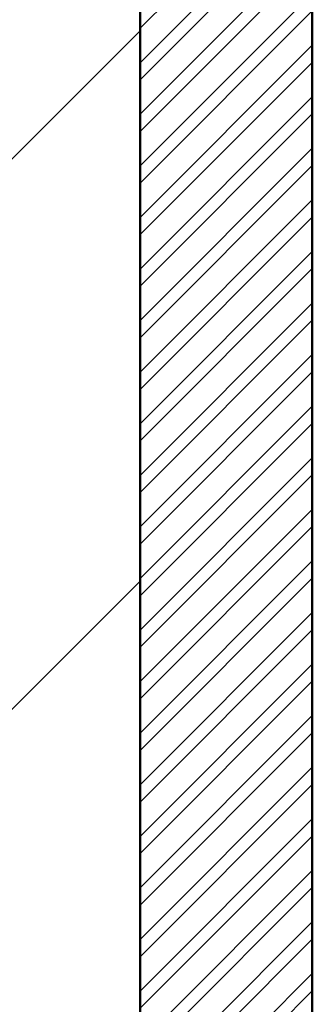
# Model space of a CAD drawing. Units: inches. Extents: x 3590 to 5167, y 65 to 1917.
# Tile 61 of 100: x 5065 to 5080, y 1558 to 1609. Entities that reach past the tile are written whole.
import ezdxf

# ---------------------------------------------------------------- set-up
doc = ezdxf.new("R2010")
doc.units = ezdxf.units.IN
for name, color, linetype, lineweight in [('A-FLOR-PATT', 8, 'Continuous', 13), ('A-WALL', 7, 'Continuous', 50), ('A-WALL-PATT', 251, 'Continuous', 13)]:
    doc.layers.add(name, color=color, linetype=linetype, lineweight=lineweight)

msp = doc.modelspace()

# ---------------------------------------------------------------- hatches: boundary and pattern name
at = {"layer": 'A-FLOR-PATT', "transparency": 33554687}
h = msp.add_hatch(dxfattribs=at)
h.set_pattern_fill('AR-HBONE', color=256, scale=0.2)
h.set_pattern_definition([(45, (-588.972, 0), (0, 28.73682), [60.96, -20.32]), (135, (-574.604, 14.368), (3e-15, 28.73682), [60.96, -20.32])])
h.paths.add_polyline_path([(5071.274, 1796.999), (4933.274, 1796.999), (4933.274, 1753.999), (4962.774, 1753.999, -0.414214), (4928.774, 1719.999), (4933.274, 1718.999), (4933.274, 1334.999), (5071.274, 1334.999)])
h.paths.add_polyline_path([(4951.78, 1521.077), (4951.715, 1521.04), (4951.563, 1520.895)], flags=16)
h.paths.add_polyline_path([(4952.267, 1521.376), (4952.198, 1521.371), (4952.198, 1521.356)], flags=0)
h.paths.add_polyline_path([(4967.051, 1529.728), (4965.231, 1528.694), (4963.411, 1527.714), (4961.756, 1526.851), (4963.589, 1527.449), (4964.036, 1527.478), (4962.975, 1527.249), (4961.76, 1526.852), (4959.792, 1525.834), (4958.005, 1524.895), (4956.24, 1523.93), (4954.504, 1522.919), (4954.129, 1522.682), (4953.361, 1521.997), (4953.366, 1521.998), (4953.605, 1522.064), (4955.106, 1522.761), (4956.921, 1523.434), (4958.678, 1523.915), (4960.358, 1524.2), (4961.945, 1524.286), (4964.171, 1524.108), (4965.958, 1523.309), (4963.863, 1522.976), (4965.187, 1522.499), (4963.366, 1522.497), (4961.545, 1522.487), (4959.764, 1522.461), (4958.304, 1522.419), (4957.974, 1522.388), (4956.307, 1522.232), (4954.718, 1522.071), (4953.251, 1521.899), (4953.525, 1521.623), (4954.331, 1521.379), (4956.243, 1521.23), (4958.039, 1520.93), (4959.684, 1520.483), (4961.16, 1519.896), (4963.107, 1518.8), (4964.393, 1517.325), (4962.973, 1517.726), (4964.558, 1516.661), (4965.407, 1515.708), (4963.507, 1516.322), (4961.68, 1517.005), (4959.935, 1517.745), (4958.282, 1518.528), (4956.732, 1519.343), (4955.295, 1520.175), (4954.672, 1520.572), (4954.513, 1520.627), (4955.658, 1519.318), (4956.703, 1517.982), (4957.644, 1516.647), (4958.485, 1515.334), (4959.55, 1513.524), (4960.438, 1511.769), (4958.841, 1513.62), (4957.452, 1515.325), (4955.819, 1517.459), (4956.665, 1515.448), (4957.111, 1513.923), (4957.447, 1511.714), (4957.076, 1509.793), (4956.538, 1511.11), (4955.992, 1512.569), (4955.444, 1514.125), (4954.898, 1515.735), (4954.357, 1517.356), (4953.824, 1518.943), (4953.305, 1520.452), (4953.065, 1521.116), (4952.971, 1521.146), (4952.949, 1521.086), (4952.73, 1520.199), (4953.37, 1518.024), (4953.757, 1516.373), (4954.051, 1514.765), (4954.264, 1513.221), (4954.471, 1511.131), (4954.497, 1510.402), (4954.409, 1511.76), (4954.264, 1513.221), (4954.051, 1514.765), (4953.757, 1516.373), (4953.37, 1518.024), (4952.877, 1519.698), (4952.716, 1520.141), (4952.533, 1519.059), (4952.374, 1517.789), (4952.219, 1516.312), (4952.046, 1514.6), (4951.833, 1512.626), (4951.557, 1510.363), (4951.203, 1512.168), (4950.852, 1514.339), (4950.985, 1516.376), (4951.66, 1518.286), (4952.593, 1520.481), (4952.357, 1521.13), (4951.855, 1520.328), (4950.839, 1518.908), (4949.777, 1517.587), (4948.916, 1516.617), (4948.111, 1515.256), (4947.089, 1513.554), (4945.889, 1511.615), (4946.326, 1513.402), (4946.562, 1514.249), (4945.528, 1513.327), (4944.581, 1512.531), (4946.018, 1514.508), (4947.204, 1516.048), (4947.893, 1517.313), (4949.307, 1518.764), (4950.414, 1519.767), (4950.451, 1519.806), (4952.267, 1521.376), (4951.645, 1521.493), (4950.404, 1521.18), (4948.044, 1520.359), (4946.119, 1519.452), (4944.572, 1518.475), (4943.35, 1517.443), (4941.997, 1515.92), (4941.661, 1515.275), (4942.813, 1516.99), (4944.572, 1518.475), (4946.119, 1519.452), (4948.044, 1520.359), (4950.404, 1521.18), (4951.645, 1521.493), (4949.647, 1521.868), (4948.6, 1521.756), (4947.126, 1521.57), (4945.42, 1521.348), (4943.45, 1521.105), (4941.183, 1520.856), (4942.86, 1521.613), (4943.873, 1522.03), (4942.952, 1521.909), (4941.41, 1521.485), (4939.543, 1520.67), (4938.968, 1520.226), (4940.733, 1521.299), (4942.952, 1521.909), (4943.702, 1522.008), (4945.894, 1522.7), (4947.565, 1522.714), (4948.921, 1522.566), (4951.131, 1522.183), (4950.971, 1522.297), (4948.129, 1523.006), (4946.035, 1523.707), (4944.232, 1524.521), (4942.707, 1525.461), (4941.444, 1526.537), (4940.43, 1527.761), (4939.649, 1529.143), (4941.421, 1528.122), (4943.147, 1527.132), (4944.841, 1526.175), (4946.514, 1525.25), (4948.179, 1524.359), (4948.365, 1524.263), (4946.475, 1526.045), (4945.181, 1527.54), (4944.19, 1529.033), (4943.496, 1530.54), (4943.278, 1531.36), (4942.498, 1531.919), (4943.114, 1531.762), (4942.959, 1533.659), (4944.14, 1531.989), (4944.612, 1531.323), (4946.202, 1530.463), (4947.486, 1529.509), (4948.79, 1528.226), (4950.368, 1526.237), (4949.485, 1528.155), (4948.851, 1530.123), (4948.491, 1532.041), (4948.381, 1533.918), (4948.501, 1535.76), (4948.827, 1537.573), (4949.418, 1535.565), (4949.957, 1533.569), (4950.464, 1531.586), (4950.961, 1529.617), (4951.391, 1527.954), (4951.724, 1530.687), (4952.201, 1532.58), (4952.889, 1534.33), (4953.77, 1535.951), (4954.827, 1537.46), (4954.521, 1535.39), (4954.273, 1533.937), (4955.58, 1535.663), (4956.748, 1536.739), (4956.159, 1534.78), (4955.589, 1532.873), (4955.043, 1531.006), (4954.525, 1529.166), (4954.038, 1527.341), (4953.638, 1525.733), (4953.611, 1525.586), (4953.398, 1524.166), (4953.382, 1524.009), (4954.07, 1525.476), (4954.912, 1527.022), (4956.136, 1528.894), (4957.847, 1530.577), (4959.376, 1531.54), (4958.256, 1530.104), (4957.143, 1528.663), (4956.066, 1527.243), (4955.056, 1525.871), (4954.141, 1524.571), (4953.352, 1523.372), (4953.311, 1523.303), (4953.273, 1522.925), (4953.261, 1522.382), (4954.103, 1523.373), (4954.63, 1524.284), (4955.961, 1526.358), (4957.23, 1528.13), (4958.421, 1529.609), (4960.037, 1531.368), (4961.374, 1532.375), (4962.101, 1532.77), (4961.07, 1531.061), (4959.987, 1529.438), (4958.869, 1527.908), (4958.15, 1527.007), (4959.803, 1528.003), (4961.589, 1528.793), (4963.391, 1529.328), (4965.211, 1529.632)], flags=16)
h.paths.add_polyline_path([(4962.944, 1523.182), (4961.107, 1523.422), (4960.392, 1523.362), (4962.35, 1523.331)], flags=0)
h.paths.add_polyline_path([(5049.541, 1584.551), (5049.476, 1584.515), (5049.325, 1584.37)], flags=16)
h.paths.add_polyline_path([(5050.028, 1584.851), (5049.959, 1584.845), (5049.959, 1584.83)], flags=0)
h.paths.add_polyline_path([(5042.333, 1581.949), (5043.88, 1582.926), (5045.806, 1583.833), (5048.165, 1584.654), (5049.406, 1584.967), (5047.408, 1585.342), (5046.361, 1585.231), (5044.888, 1585.044), (5043.181, 1584.822), (5041.211, 1584.579), (5038.944, 1584.33), (5040.622, 1585.087), (5041.634, 1585.504), (5040.713, 1585.383), (5039.171, 1584.959), (5037.304, 1584.144), (5036.729, 1583.7), (5038.494, 1584.773), (5040.713, 1585.383), (5041.463, 1585.482), (5043.655, 1586.174), (5045.326, 1586.188), (5046.682, 1586.04), (5048.893, 1585.657), (5048.732, 1585.771), (5045.891, 1586.48), (5043.796, 1587.181), (5041.994, 1587.996), (5040.468, 1588.935), (5039.205, 1590.011), (5038.191, 1591.235), (5037.41, 1592.617), (5039.182, 1591.596), (5040.909, 1590.607), (5042.602, 1589.649), (5044.275, 1588.724), (5045.94, 1587.833), (5046.126, 1587.738), (5044.237, 1589.519), (5042.942, 1591.015), (5041.952, 1592.508), (5041.257, 1594.014), (5041.039, 1594.834), (5040.26, 1595.393), (5040.875, 1595.237), (5040.721, 1597.133), (5041.901, 1595.463), (5042.373, 1594.798), (5043.963, 1593.938), (5045.247, 1592.983), (5046.552, 1591.701), (5048.129, 1589.712), (5047.247, 1591.63), (5046.613, 1593.597), (5046.252, 1595.515), (5046.142, 1597.392), (5046.262, 1599.234), (5046.588, 1601.047), (5047.179, 1599.039), (5047.718, 1597.043), (5048.225, 1595.06), (5048.722, 1593.091), (5049.152, 1591.429), (5049.485, 1594.161), (5049.962, 1596.054), (5050.65, 1597.804), (5051.532, 1599.425), (5052.589, 1600.934), (5052.283, 1598.864), (5052.034, 1597.411), (5053.341, 1599.137), (5054.509, 1600.213), (5053.92, 1598.254), (5053.35, 1596.348), (5052.805, 1594.48), (5052.286, 1592.64), (5051.799, 1590.815), (5051.4, 1589.207), (5051.373, 1589.06), (5051.159, 1587.64), (5051.143, 1587.483), (5051.831, 1588.95), (5052.673, 1590.496), (5053.898, 1592.368), (5055.608, 1594.051), (5057.137, 1595.014), (5056.017, 1593.578), (5054.904, 1592.137), (5053.828, 1590.717), (5052.817, 1589.345), (5051.902, 1588.046), (5051.113, 1586.846), (5051.072, 1586.777), (5051.034, 1586.399), (5051.022, 1585.856), (5051.864, 1586.847), (5052.391, 1587.758), (5053.723, 1589.832), (5054.991, 1591.604), (5056.182, 1593.083), (5057.798, 1594.842), (5059.135, 1595.849), (5059.863, 1596.244), (5058.831, 1594.535), (5057.749, 1592.912), (5056.63, 1591.382), (5055.912, 1590.482), (5057.564, 1591.477), (5059.35, 1592.267), (5061.152, 1592.802), (5062.972, 1593.106), (5064.812, 1593.203), (5062.992, 1592.169), (5061.172, 1591.188), (5059.518, 1590.325), (5061.35, 1590.924), (5061.797, 1590.952), (5060.737, 1590.723), (5059.521, 1590.326), (5057.553, 1589.308), (5055.766, 1588.369), (5054.002, 1587.404), (5052.265, 1586.393), (5051.891, 1586.156), (5051.122, 1585.471), (5051.127, 1585.472), (5051.366, 1585.538), (5052.867, 1586.235), (5054.682, 1586.908), (5056.439, 1587.389), (5058.12, 1587.675), (5059.706, 1587.76), (5061.933, 1587.583), (5063.719, 1586.783), (5061.624, 1586.45), (5062.949, 1585.973), (5061.127, 1585.971), (5059.307, 1585.961), (5057.525, 1585.935), (5056.065, 1585.893), (5055.735, 1585.862), (5054.068, 1585.707), (5052.479, 1585.546), (5051.012, 1585.373), (5051.286, 1585.097), (5052.092, 1584.853), (5054.004, 1584.704), (5055.8, 1584.404), (5057.446, 1583.958), (5058.921, 1583.37), (5060.868, 1582.274), (5062.154, 1580.799), (5060.734, 1581.2), (5062.32, 1580.135), (5063.168, 1579.182), (5061.269, 1579.796), (5059.441, 1580.479), (5057.696, 1581.219), (5056.043, 1582.003), (5054.493, 1582.817), (5053.057, 1583.649), (5052.433, 1584.047), (5052.274, 1584.101), (5053.42, 1582.793), (5054.464, 1581.457), (5055.405, 1580.121), (5056.247, 1578.809), (5057.311, 1576.998), (5058.199, 1575.244), (5056.602, 1577.094), (5055.213, 1578.799), (5053.58, 1580.933), (5054.427, 1578.922), (5054.872, 1577.397), (5055.208, 1575.189), (5054.838, 1573.267), (5054.299, 1574.584), (5053.754, 1576.043), (5053.206, 1577.599), (5052.659, 1579.209), (5052.118, 1580.83), (5051.585, 1582.417), (5051.066, 1583.927), (5050.826, 1584.59), (5050.733, 1584.62), (5050.711, 1584.561), (5050.491, 1583.673), (5051.131, 1581.498), (5051.518, 1579.847), (5051.813, 1578.24), (5052.026, 1576.695), (5052.233, 1574.605), (5052.258, 1573.876), (5052.17, 1575.234), (5052.026, 1576.695), (5051.813, 1578.24), (5051.518, 1579.847), (5051.131, 1581.498), (5050.638, 1583.172), (5050.477, 1583.615), (5050.294, 1582.533), (5050.136, 1581.263), (5049.981, 1579.786), (5049.807, 1578.074), (5049.594, 1576.1), (5049.318, 1573.837), (5048.965, 1575.642), (5048.613, 1577.813), (5048.747, 1579.85), (5049.421, 1581.76), (5050.354, 1583.955), (5050.118, 1584.604), (5049.616, 1583.802), (5048.6, 1582.382), (5047.538, 1581.061), (5046.677, 1580.091), (5045.872, 1578.73), (5044.85, 1577.028), (5043.651, 1575.089), (5044.087, 1576.877), (5044.324, 1577.723), (5043.289, 1576.801), (5042.342, 1576.005), (5043.779, 1577.982), (5044.966, 1579.522), (5045.655, 1580.787), (5047.068, 1582.239), (5048.175, 1583.241), (5048.213, 1583.28), (5050.028, 1584.851), (5049.406, 1584.967), (5048.165, 1584.654), (5045.806, 1583.833), (5043.88, 1582.926), (5042.333, 1581.949), (5041.111, 1580.917), (5039.758, 1579.394), (5039.423, 1578.749), (5040.575, 1580.464)], flags=16)
h.paths.add_polyline_path([(4954.799, 1533.12), (4954.262, 1532.079), (4953.831, 1530.935), (4953.505, 1529.636), (4953.283, 1528.133), (4953.167, 1526.376), (4953.156, 1524.315), (4953.277, 1521.236), (4952.802, 1521.842), (4951.557, 1521.998), (4950.976, 1521.961), (4952.661, 1521.941), (4952.802, 1521.842), (4953.152, 1523.593), (4953.167, 1526.376), (4953.283, 1528.133), (4953.609, 1530.346), (4954.456, 1532.592)], flags=0)
h.paths.add_polyline_path([(5050.563, 1585.316), (5049.318, 1585.472), (5048.737, 1585.435), (5050.422, 1585.415), (5050.563, 1585.316), (5050.914, 1587.067), (5050.928, 1589.851), (5051.045, 1591.607), (5051.371, 1593.82), (5052.217, 1596.066), (5052.56, 1596.594), (5052.024, 1595.554), (5051.592, 1594.409), (5051.266, 1593.11), (5051.045, 1591.607), (5050.928, 1589.851), (5050.918, 1587.789), (5051.038, 1584.71)], flags=0)
h.paths.add_polyline_path([(5058.153, 1586.836), (5060.111, 1586.805), (5060.705, 1586.656), (5058.868, 1586.896)], flags=0)
h.paths.add_polyline_path([(5049.541, 1430.936), (5049.476, 1430.9), (5049.325, 1430.755)], flags=16)
h.paths.add_polyline_path([(5050.028, 1431.236), (5049.959, 1431.231), (5049.959, 1431.215)], flags=0)
h.paths.add_polyline_path([(5046.588, 1447.432), (5047.179, 1445.425), (5047.718, 1443.429), (5048.225, 1441.446), (5048.722, 1439.476), (5049.152, 1437.814), (5049.485, 1440.546), (5049.962, 1442.439), (5050.65, 1444.189), (5051.532, 1445.811), (5052.589, 1447.319), (5052.283, 1445.249), (5052.034, 1443.796), (5053.341, 1445.522), (5054.509, 1446.598), (5053.92, 1444.64), (5053.35, 1442.733), (5052.805, 1440.865), (5052.286, 1439.025), (5051.799, 1437.201), (5051.4, 1435.592), (5051.373, 1435.445), (5051.159, 1434.025), (5051.143, 1433.868), (5051.831, 1435.335), (5052.673, 1436.881), (5053.898, 1438.753), (5055.608, 1440.436), (5057.137, 1441.4), (5056.017, 1439.963), (5054.904, 1438.522), (5053.828, 1437.102), (5052.817, 1435.73), (5051.902, 1434.431), (5051.113, 1433.231), (5051.072, 1433.162), (5051.034, 1432.784), (5051.022, 1432.242), (5051.864, 1433.232), (5052.391, 1434.143), (5053.723, 1436.217), (5054.991, 1437.989), (5056.182, 1439.468), (5057.798, 1441.227), (5059.135, 1442.235), (5059.863, 1442.629), (5058.831, 1440.921), (5057.749, 1439.298), (5056.63, 1437.767), (5055.912, 1436.867), (5057.564, 1437.863), (5059.35, 1438.652), (5061.152, 1439.187), (5062.972, 1439.491), (5064.812, 1439.588), (5062.992, 1438.554), (5061.172, 1437.573), (5059.518, 1436.71), (5061.35, 1437.309), (5061.797, 1437.337), (5060.737, 1437.108), (5059.521, 1436.711), (5057.553, 1435.693), (5055.766, 1434.754), (5054.002, 1433.789), (5052.265, 1432.778), (5051.891, 1432.541), (5051.122, 1431.856), (5051.127, 1431.857), (5051.366, 1431.923), (5052.867, 1432.62), (5054.682, 1433.293), (5056.439, 1433.775), (5058.12, 1434.06), (5059.706, 1434.145), (5061.933, 1433.968), (5063.719, 1433.168), (5061.624, 1432.835), (5062.949, 1432.358), (5061.127, 1432.357), (5059.307, 1432.346), (5057.525, 1432.32), (5056.065, 1432.278), (5055.735, 1432.248), (5054.068, 1432.092), (5052.479, 1431.931), (5051.012, 1431.759), (5051.286, 1431.482), (5052.092, 1431.238), (5054.004, 1431.089), (5055.8, 1430.789), (5057.446, 1430.343), (5058.921, 1429.755), (5060.868, 1428.66), (5062.154, 1427.185), (5060.734, 1427.585), (5062.32, 1426.52), (5063.168, 1425.567), (5061.269, 1426.181), (5059.441, 1426.865), (5057.696, 1427.604), (5056.043, 1428.388), (5054.493, 1429.202), (5053.057, 1430.034), (5052.433, 1430.432), (5052.274, 1430.487), (5053.42, 1429.178), (5054.464, 1427.842), (5055.405, 1426.506), (5056.247, 1425.194), (5057.311, 1423.383), (5058.199, 1421.629), (5056.602, 1423.479), (5055.213, 1425.184), (5053.58, 1427.318), (5054.427, 1425.307), (5054.872, 1423.782), (5055.208, 1421.574), (5054.838, 1419.652), (5054.299, 1420.97), (5053.754, 1422.428), (5053.206, 1423.984), (5052.659, 1425.595), (5052.118, 1427.215), (5051.585, 1428.802), (5051.066, 1430.312), (5050.826, 1430.975), (5050.733, 1431.005), (5050.711, 1430.946), (5050.491, 1430.058), (5051.131, 1427.883), (5051.518, 1426.232), (5051.813, 1424.625), (5052.026, 1423.081), (5052.233, 1420.991), (5052.258, 1420.261), (5052.17, 1421.619), (5052.026, 1423.081), (5051.813, 1424.625), (5051.518, 1426.232), (5051.131, 1427.883), (5050.638, 1429.558), (5050.477, 1430.001), (5050.294, 1428.918), (5050.136, 1427.648), (5049.981, 1426.171), (5049.807, 1424.459), (5049.594, 1422.485), (5049.318, 1420.222), (5048.965, 1422.028), (5048.613, 1424.199), (5048.747, 1426.235), (5049.421, 1428.146), (5050.354, 1430.34), (5050.118, 1430.989), (5049.616, 1430.187), (5048.6, 1428.768), (5047.538, 1427.446), (5046.677, 1426.477), (5045.872, 1425.116), (5044.85, 1423.413), (5043.651, 1421.474), (5044.087, 1423.262), (5044.324, 1424.109), (5043.289, 1423.186), (5042.342, 1422.391), (5043.779, 1424.368), (5044.966, 1425.907), (5045.655, 1427.173), (5047.068, 1428.624), (5048.175, 1429.627), (5048.213, 1429.666), (5050.028, 1431.236), (5049.406, 1431.353), (5048.165, 1431.039), (5045.806, 1430.218), (5043.88, 1429.311), (5042.333, 1428.334), (5041.111, 1427.302), (5039.758, 1425.779), (5039.423, 1425.134), (5040.575, 1426.849), (5042.333, 1428.334), (5043.88, 1429.311), (5045.806, 1430.218), (5048.165, 1431.039), (5049.406, 1431.353), (5047.408, 1431.727), (5046.361, 1431.616), (5044.888, 1431.429), (5043.181, 1431.207), (5041.211, 1430.964), (5038.944, 1430.715), (5040.622, 1431.472), (5041.634, 1431.89), (5040.713, 1431.769), (5039.171, 1431.345), (5037.304, 1430.53), (5036.729, 1430.085), (5038.494, 1431.158), (5040.713, 1431.769), (5041.463, 1431.867), (5043.655, 1432.559), (5045.326, 1432.573), (5046.682, 1432.425), (5048.893, 1432.042), (5048.732, 1432.156), (5045.891, 1432.865), (5043.796, 1433.566), (5041.994, 1434.381), (5040.468, 1435.321), (5039.205, 1436.396), (5038.191, 1437.62), (5037.41, 1439.002), (5039.182, 1437.982), (5040.909, 1436.992), (5042.602, 1436.034), (5044.275, 1435.109), (5045.94, 1434.218), (5046.126, 1434.123), (5044.237, 1435.904), (5042.942, 1437.4), (5041.952, 1438.893), (5041.257, 1440.399), (5041.039, 1441.219), (5040.26, 1441.778), (5040.875, 1441.622), (5040.721, 1443.518), (5041.901, 1441.848), (5042.373, 1441.183), (5043.963, 1440.323), (5045.247, 1439.369), (5046.552, 1438.086), (5048.129, 1436.097), (5047.247, 1438.015), (5046.613, 1439.982), (5046.252, 1441.901), (5046.142, 1443.778), (5046.262, 1445.619)], flags=16)
h.paths.add_polyline_path([(5052.382, 1444.255), (5051.623, 1442.78), (5052.024, 1441.939), (5052.56, 1442.98)], flags=0)
h.paths.add_polyline_path([(5050.563, 1431.701), (5049.318, 1431.857), (5048.737, 1431.821), (5050.422, 1431.8)], flags=0)
h.paths.add_polyline_path([(5058.153, 1433.221), (5060.111, 1433.19), (5060.705, 1433.041), (5058.868, 1433.281)], flags=0)
h.paths.add_polyline_path([(5049.541, 1352.285), (5049.476, 1352.249), (5049.325, 1352.104)], flags=16)
h.paths.add_polyline_path([(5050.028, 1352.585), (5049.959, 1352.58), (5049.959, 1352.564)], flags=0)
h.paths.add_polyline_path([(5046.588, 1368.781), (5047.179, 1366.774), (5047.718, 1364.778), (5048.225, 1362.795), (5048.722, 1360.825), (5049.152, 1359.163), (5049.485, 1361.896), (5049.962, 1363.789), (5050.65, 1365.538), (5051.532, 1367.16), (5052.589, 1368.669), (5052.283, 1366.598), (5052.034, 1365.145), (5053.341, 1366.871), (5054.509, 1367.947), (5053.92, 1365.989), (5053.35, 1364.082), (5052.805, 1362.214), (5052.286, 1360.374), (5051.799, 1358.55), (5051.4, 1356.942), (5051.373, 1356.794), (5051.159, 1355.374), (5051.143, 1355.218), (5051.831, 1356.684), (5052.673, 1358.23), (5053.898, 1360.102), (5055.608, 1361.786), (5057.137, 1362.749), (5056.017, 1361.313), (5054.904, 1359.872), (5053.828, 1358.452), (5052.817, 1357.079), (5051.902, 1355.78), (5051.113, 1354.581), (5051.072, 1354.512), (5051.034, 1354.133), (5051.022, 1353.591), (5051.864, 1354.581), (5052.391, 1355.492), (5053.723, 1357.566), (5054.991, 1359.338), (5056.182, 1360.817), (5057.798, 1362.577), (5059.135, 1363.584), (5059.863, 1363.979), (5058.831, 1362.27), (5057.749, 1360.647), (5056.63, 1359.117), (5055.912, 1358.216), (5057.564, 1359.212), (5059.35, 1360.001), (5061.152, 1360.536), (5062.972, 1360.841), (5064.812, 1360.937), (5062.992, 1359.903), (5061.172, 1358.923), (5059.518, 1358.059), (5061.35, 1358.658), (5061.797, 1358.687), (5060.737, 1358.458), (5059.521, 1358.061), (5057.553, 1357.043), (5055.766, 1356.103), (5054.002, 1355.138), (5052.265, 1354.127), (5051.891, 1353.89), (5051.122, 1353.206), (5051.127, 1353.206), (5051.366, 1353.272), (5052.867, 1353.969), (5054.682, 1354.643), (5056.439, 1355.124), (5058.12, 1355.409), (5059.706, 1355.495), (5061.933, 1355.317), (5063.719, 1354.518), (5061.624, 1354.184), (5062.949, 1353.708), (5061.127, 1353.706), (5059.307, 1353.695), (5057.525, 1353.669), (5056.065, 1353.627), (5055.735, 1353.597), (5054.068, 1353.441), (5052.479, 1353.28), (5051.012, 1353.108), (5051.286, 1352.831), (5052.092, 1352.587), (5054.004, 1352.439), (5055.8, 1352.138), (5057.446, 1351.692), (5058.921, 1351.104), (5060.868, 1350.009), (5062.154, 1348.534), (5060.734, 1348.935), (5062.32, 1347.869), (5063.168, 1346.916), (5061.269, 1347.53), (5059.441, 1348.214), (5057.696, 1348.954), (5056.043, 1349.737), (5054.493, 1350.551), (5053.057, 1351.383), (5052.433, 1351.781), (5052.274, 1351.836), (5053.42, 1350.527), (5054.464, 1349.191), (5055.405, 1347.855), (5056.247, 1346.543), (5057.311, 1344.733), (5058.199, 1342.978), (5056.602, 1344.828), (5055.213, 1346.534), (5053.58, 1348.667), (5054.427, 1346.656), (5054.872, 1345.132), (5055.208, 1342.923), (5054.838, 1341.002), (5054.299, 1342.319), (5053.754, 1343.778), (5053.206, 1345.334), (5052.659, 1346.944), (5052.118, 1348.564), (5051.585, 1350.151), (5051.066, 1351.661), (5050.826, 1352.324), (5050.733, 1352.355), (5050.711, 1352.295), (5050.491, 1351.408), (5051.131, 1349.232), (5051.518, 1347.581), (5051.813, 1345.974), (5052.026, 1344.43), (5052.233, 1342.34), (5052.258, 1341.61), (5052.17, 1342.969), (5052.026, 1344.43), (5051.813, 1345.974), (5051.518, 1347.581), (5051.131, 1349.232), (5050.638, 1350.907), (5050.477, 1351.35), (5050.294, 1350.267), (5050.136, 1348.997), (5049.981, 1347.52), (5049.807, 1345.809), (5049.594, 1343.835), (5049.318, 1341.571), (5048.965, 1343.377), (5048.613, 1345.548), (5048.747, 1347.585), (5049.421, 1349.495), (5050.354, 1351.689), (5050.118, 1352.339), (5049.616, 1351.536), (5048.6, 1350.117), (5047.538, 1348.795), (5046.677, 1347.826), (5045.872, 1346.465), (5044.85, 1344.763), (5043.651, 1342.824), (5044.087, 1344.611), (5044.324, 1345.458), (5043.289, 1344.535), (5042.342, 1343.74), (5043.779, 1345.717), (5044.966, 1347.256), (5045.655, 1348.522), (5047.068, 1349.973), (5048.175, 1350.976), (5048.213, 1351.015), (5050.028, 1352.585), (5049.406, 1352.702), (5048.165, 1352.388), (5045.806, 1351.567), (5043.88, 1350.661), (5042.333, 1349.683), (5041.111, 1348.651), (5039.758, 1347.128), (5039.423, 1346.483), (5040.575, 1348.198), (5042.333, 1349.683), (5043.88, 1350.661), (5045.806, 1351.567), (5048.165, 1352.388), (5049.406, 1352.702), (5047.408, 1353.076), (5046.361, 1352.965), (5044.888, 1352.779), (5043.181, 1352.556), (5041.211, 1352.313), (5038.944, 1352.065), (5040.622, 1352.821), (5041.634, 1353.239), (5040.713, 1353.118), (5039.171, 1352.694), (5037.304, 1351.879), (5036.729, 1351.434), (5038.494, 1352.508), (5040.713, 1353.118), (5041.463, 1353.216), (5043.655, 1353.909), (5045.326, 1353.923), (5046.682, 1353.774), (5048.893, 1353.391), (5048.732, 1353.506), (5045.891, 1354.214), (5043.796, 1354.915), (5041.994, 1355.73), (5040.468, 1356.67), (5039.205, 1357.746), (5038.191, 1358.969), (5037.41, 1360.352), (5039.182, 1359.331), (5040.909, 1358.341), (5042.602, 1357.383), (5044.275, 1356.458), (5045.94, 1355.567), (5046.126, 1355.472), (5044.237, 1357.253), (5042.942, 1358.749), (5041.952, 1360.242), (5041.257, 1361.748), (5041.039, 1362.568), (5040.26, 1363.128), (5040.875, 1362.971), (5040.721, 1364.867), (5041.901, 1363.197), (5042.373, 1362.532), (5043.963, 1361.672), (5045.247, 1360.718), (5046.552, 1359.435), (5048.129, 1357.446), (5047.247, 1359.364), (5046.613, 1361.331), (5046.252, 1363.25), (5046.142, 1365.127), (5046.262, 1366.969)], flags=16)
h.paths.add_polyline_path([(5052.382, 1365.604), (5051.623, 1364.129), (5052.024, 1363.288), (5052.56, 1364.329)], flags=0)
h.paths.add_polyline_path([(4951.78, 1698.041), (4951.715, 1698.005), (4951.563, 1697.859)], flags=16)
h.paths.add_polyline_path([(4952.267, 1698.341), (4952.198, 1698.335), (4952.198, 1698.32)], flags=0)
h.paths.add_polyline_path([(4957.076, 1686.757), (4956.538, 1688.074), (4955.992, 1689.533), (4955.444, 1691.089), (4954.898, 1692.699), (4954.357, 1694.32), (4953.824, 1695.907), (4953.305, 1697.417), (4953.065, 1698.08), (4952.971, 1698.11), (4952.949, 1698.051), (4952.73, 1697.163), (4953.37, 1694.988), (4953.757, 1693.337), (4954.051, 1691.729), (4954.264, 1690.185), (4954.471, 1688.095), (4954.497, 1687.366), (4954.409, 1688.724), (4954.264, 1690.185), (4954.051, 1691.729), (4953.757, 1693.337), (4953.37, 1694.988), (4952.877, 1696.662), (4952.716, 1697.105), (4952.533, 1696.023), (4952.374, 1694.753), (4952.219, 1693.276), (4952.046, 1691.564), (4951.833, 1689.59), (4951.557, 1687.327), (4951.203, 1689.132), (4950.852, 1691.303), (4950.985, 1693.34), (4951.66, 1695.25), (4952.593, 1697.445), (4952.357, 1698.094), (4951.855, 1697.292), (4950.839, 1695.872), (4949.777, 1694.551), (4948.916, 1693.581), (4948.111, 1692.22), (4947.089, 1690.518), (4945.889, 1688.579), (4946.326, 1690.366), (4946.562, 1691.213), (4945.528, 1690.291), (4944.581, 1689.495), (4946.018, 1691.472), (4947.204, 1693.012), (4947.893, 1694.277), (4949.307, 1695.729), (4950.414, 1696.731), (4950.451, 1696.77), (4952.267, 1698.341), (4951.645, 1698.457), (4950.404, 1698.144), (4948.044, 1697.323), (4946.119, 1696.416), (4944.572, 1695.439), (4943.35, 1694.407), (4941.997, 1692.884), (4941.661, 1692.239), (4942.813, 1693.954), (4944.572, 1695.439), (4946.119, 1696.416), (4948.044, 1697.323), (4950.404, 1698.144), (4951.645, 1698.457), (4949.647, 1698.832), (4948.6, 1698.72), (4947.126, 1698.534), (4945.42, 1698.312), (4943.45, 1698.069), (4941.183, 1697.82), (4942.86, 1698.577), (4943.873, 1698.994), (4942.952, 1698.873), (4941.41, 1698.449), (4939.543, 1697.634), (4938.968, 1697.19), (4940.733, 1698.263), (4942.952, 1698.873), (4943.702, 1698.972), (4945.894, 1699.664), (4947.565, 1699.678), (4948.921, 1699.53), (4951.131, 1699.147), (4950.971, 1699.261), (4948.129, 1699.97), (4946.035, 1700.671), (4944.232, 1701.486), (4942.707, 1702.425), (4941.444, 1703.501), (4940.43, 1704.725), (4939.649, 1706.107), (4941.421, 1705.086), (4943.147, 1704.097), (4944.841, 1703.139), (4946.514, 1702.214), (4948.179, 1701.323), (4948.365, 1701.227), (4946.475, 1703.009), (4945.181, 1704.505), (4944.19, 1705.997), (4943.496, 1707.504), (4943.278, 1708.324), (4942.498, 1708.883), (4943.114, 1708.727), (4942.959, 1710.623), (4944.14, 1708.953), (4944.612, 1708.287), (4946.202, 1707.428), (4947.486, 1706.473), (4948.79, 1705.191), (4950.368, 1703.202), (4949.485, 1705.12), (4948.851, 1707.087), (4948.491, 1709.005), (4948.381, 1710.882), (4948.501, 1712.724), (4948.827, 1714.537), (4949.418, 1712.529), (4949.957, 1710.533), (4950.464, 1708.55), (4950.961, 1706.581), (4951.391, 1704.919), (4951.724, 1707.651), (4952.201, 1709.544), (4952.889, 1711.294), (4953.77, 1712.915), (4954.827, 1714.424), (4954.521, 1712.354), (4954.273, 1710.901), (4955.58, 1712.627), (4956.748, 1713.703), (4956.159, 1711.744), (4955.589, 1709.837), (4955.043, 1707.97), (4954.525, 1706.13), (4954.038, 1704.305), (4953.638, 1702.697), (4953.611, 1702.55), (4953.398, 1701.13), (4953.382, 1700.973), (4954.07, 1702.44), (4954.912, 1703.986), (4956.136, 1705.858), (4957.847, 1707.541), (4959.376, 1708.504), (4958.256, 1707.068), (4957.143, 1705.627), (4956.066, 1704.207), (4955.056, 1702.835), (4954.141, 1701.536), (4953.352, 1700.336), (4953.311, 1700.267), (4953.273, 1699.889), (4953.261, 1699.346), (4954.103, 1700.337), (4954.63, 1701.248), (4955.961, 1703.322), (4957.23, 1705.094), (4958.421, 1706.573), (4960.037, 1708.332), (4961.374, 1709.339), (4962.101, 1709.734), (4961.07, 1708.025), (4959.987, 1706.402), (4958.869, 1704.872), (4958.15, 1703.972), (4959.803, 1704.967), (4961.589, 1705.757), (4963.391, 1706.292), (4965.211, 1706.596), (4967.051, 1706.692), (4965.231, 1705.659), (4963.411, 1704.678), (4961.756, 1703.815), (4963.589, 1704.413), (4964.036, 1704.442), (4962.975, 1704.213), (4961.76, 1703.816), (4959.792, 1702.798), (4958.005, 1701.859), (4956.24, 1700.894), (4954.504, 1699.883), (4954.129, 1699.646), (4953.361, 1698.961), (4953.366, 1698.962), (4953.605, 1699.028), (4955.106, 1699.725), (4956.921, 1700.398), (4958.678, 1700.879), (4960.358, 1701.164), (4961.945, 1701.25), (4964.171, 1701.073), (4965.958, 1700.273), (4963.863, 1699.94), (4965.187, 1699.463), (4963.366, 1699.461), (4961.545, 1699.451), (4959.764, 1699.425), (4958.304, 1699.383), (4957.974, 1699.352), (4956.307, 1699.197), (4954.718, 1699.036), (4953.251, 1698.863), (4953.525, 1698.587), (4954.331, 1698.343), (4956.243, 1698.194), (4958.039, 1697.894), (4959.684, 1697.447), (4961.16, 1696.86), (4963.107, 1695.764), (4964.393, 1694.289), (4962.973, 1694.69), (4964.558, 1693.625), (4965.407, 1692.672), (4963.507, 1693.286), (4961.68, 1693.969), (4959.935, 1694.709), (4958.282, 1695.492), (4956.732, 1696.307), (4955.295, 1697.139), (4954.672, 1697.536), (4954.513, 1697.591), (4955.658, 1696.282), (4956.703, 1694.946), (4957.644, 1693.611), (4958.485, 1692.298), (4959.55, 1690.488), (4960.438, 1688.733), (4958.841, 1690.584), (4957.452, 1692.289), (4955.819, 1694.423), (4956.665, 1692.412), (4957.111, 1690.887), (4957.447, 1688.678)], flags=16)
h.paths.add_polyline_path([(5050.563, 1353.05), (5049.318, 1353.207), (5048.737, 1353.17), (5050.422, 1353.15)], flags=0)
h.paths.add_polyline_path([(4951.78, 1351.486), (4951.715, 1351.45), (4951.563, 1351.305)], flags=16)
h.paths.add_polyline_path([(4952.267, 1351.786), (4952.198, 1351.78), (4952.198, 1351.765)], flags=0)
h.paths.add_polyline_path([(4954.827, 1367.869), (4954.521, 1365.799), (4954.273, 1364.346), (4955.58, 1366.072), (4956.748, 1367.148), (4956.159, 1365.19), (4955.589, 1363.283), (4955.043, 1361.415), (4954.525, 1359.575), (4954.038, 1357.751), (4953.638, 1356.142), (4953.611, 1355.995), (4953.398, 1354.575), (4953.382, 1354.418), (4954.07, 1355.885), (4954.912, 1357.431), (4956.136, 1359.303), (4957.847, 1360.986), (4959.376, 1361.95), (4958.256, 1360.513), (4957.143, 1359.072), (4956.066, 1357.652), (4955.056, 1356.28), (4954.141, 1354.981), (4953.352, 1353.781), (4953.311, 1353.712), (4953.273, 1353.334), (4953.261, 1352.792), (4954.103, 1353.782), (4954.63, 1354.693), (4955.961, 1356.767), (4957.23, 1358.539), (4958.421, 1360.018), (4960.037, 1361.777), (4961.374, 1362.785), (4962.101, 1363.179), (4961.07, 1361.471), (4959.987, 1359.848), (4958.869, 1358.317), (4958.15, 1357.417), (4959.803, 1358.413), (4961.589, 1359.202), (4963.391, 1359.737), (4965.211, 1360.041), (4967.051, 1360.138), (4965.231, 1359.104), (4963.411, 1358.123), (4961.756, 1357.26), (4963.589, 1357.859), (4964.036, 1357.887), (4962.975, 1357.658), (4961.76, 1357.261), (4959.792, 1356.243), (4958.005, 1355.304), (4956.24, 1354.339), (4954.504, 1353.328), (4954.129, 1353.091), (4953.361, 1352.406), (4953.366, 1352.407), (4953.605, 1352.473), (4955.106, 1353.17), (4956.921, 1353.843), (4958.678, 1354.325), (4960.358, 1354.61), (4961.945, 1354.695), (4964.171, 1354.518), (4965.958, 1353.718), (4963.863, 1353.385), (4965.187, 1352.908), (4963.366, 1352.907), (4961.545, 1352.896), (4959.764, 1352.87), (4958.304, 1352.828), (4957.974, 1352.798), (4956.307, 1352.642), (4954.718, 1352.481), (4953.251, 1352.309), (4953.525, 1352.032), (4954.331, 1351.788), (4956.243, 1351.639), (4958.039, 1351.339), (4959.684, 1350.893), (4961.16, 1350.305), (4963.107, 1349.21), (4964.393, 1347.735), (4962.973, 1348.135), (4964.558, 1347.07), (4965.407, 1346.117), (4963.507, 1346.731), (4961.68, 1347.414), (4959.935, 1348.154), (4958.282, 1348.938), (4956.732, 1349.752), (4955.295, 1350.584), (4954.672, 1350.982), (4954.513, 1351.036), (4955.658, 1349.728), (4956.703, 1348.392), (4957.644, 1347.056), (4958.485, 1345.744), (4959.55, 1343.933), (4960.438, 1342.179), (4958.841, 1344.029), (4957.452, 1345.734), (4955.819, 1347.868), (4956.665, 1345.857), (4957.111, 1344.332), (4957.447, 1342.124), (4957.076, 1340.202), (4956.538, 1341.52), (4955.992, 1342.978), (4955.444, 1344.534), (4954.898, 1346.145), (4954.357, 1347.765), (4953.824, 1349.352), (4953.305, 1350.862), (4953.065, 1351.525), (4952.971, 1351.555), (4952.949, 1351.496), (4952.73, 1350.608), (4953.37, 1348.433), (4953.757, 1346.782), (4954.051, 1345.175), (4954.264, 1343.631), (4954.471, 1341.541), (4954.497, 1340.811), (4954.409, 1342.169), (4954.264, 1343.631), (4954.051, 1345.175), (4953.757, 1346.782), (4953.37, 1348.433), (4952.877, 1350.108), (4952.716, 1350.551), (4952.533, 1349.468), (4952.374, 1348.198), (4952.219, 1346.721), (4952.046, 1345.009), (4951.833, 1343.035), (4951.557, 1340.772), (4951.203, 1342.578), (4950.852, 1344.749), (4950.985, 1346.785), (4951.66, 1348.696), (4952.593, 1350.89), (4952.357, 1351.539), (4951.855, 1350.737), (4950.839, 1349.318), (4949.777, 1347.996), (4948.916, 1347.027), (4948.111, 1345.665), (4947.089, 1343.963), (4945.889, 1342.024), (4946.326, 1343.812), (4946.562, 1344.659), (4945.528, 1343.736), (4944.581, 1342.941), (4946.018, 1344.918), (4947.204, 1346.457), (4947.893, 1347.723), (4949.307, 1349.174), (4950.414, 1350.177), (4950.451, 1350.216), (4952.267, 1351.786), (4951.645, 1351.903), (4950.404, 1351.589), (4948.044, 1350.768), (4946.119, 1349.861), (4944.572, 1348.884), (4943.35, 1347.852), (4941.997, 1346.329), (4941.661, 1345.684), (4942.813, 1347.399), (4944.572, 1348.884), (4946.119, 1349.861), (4948.044, 1350.768), (4950.404, 1351.589), (4951.645, 1351.903), (4949.647, 1352.277), (4948.6, 1352.166), (4947.126, 1351.979), (4945.42, 1351.757), (4943.45, 1351.514), (4941.183, 1351.265), (4942.86, 1352.022), (4943.873, 1352.44), (4942.952, 1352.319), (4941.41, 1351.895), (4939.543, 1351.08), (4938.968, 1350.635), (4940.733, 1351.708), (4942.952, 1352.319), (4943.702, 1352.417), (4945.894, 1353.109), (4947.565, 1353.123), (4948.921, 1352.975), (4951.131, 1352.592), (4950.971, 1352.706), (4948.129, 1353.415), (4946.035, 1354.116), (4944.232, 1354.931), (4942.707, 1355.871), (4941.444, 1356.946), (4940.43, 1358.17), (4939.649, 1359.552), (4941.421, 1358.532), (4943.147, 1357.542), (4944.841, 1356.584), (4946.514, 1355.659), (4948.179, 1354.768), (4948.365, 1354.673), (4946.475, 1356.454), (4945.181, 1357.95), (4944.19, 1359.443), (4943.496, 1360.949), (4943.278, 1361.769), (4942.498, 1362.328), (4943.114, 1362.172), (4942.959, 1364.068), (4944.14, 1362.398), (4944.612, 1361.733), (4946.202, 1360.873), (4947.486, 1359.919), (4948.79, 1358.636), (4950.368, 1356.647), (4949.485, 1358.565), (4948.851, 1360.532), (4948.491, 1362.451), (4948.381, 1364.328), (4948.501, 1366.169), (4948.827, 1367.982), (4949.418, 1365.975), (4949.957, 1363.979), (4950.464, 1361.995), (4950.961, 1360.026), (4951.391, 1358.364), (4951.724, 1361.096), (4952.201, 1362.989), (4952.889, 1364.739), (4953.77, 1366.361)], flags=16)
h.paths.add_polyline_path([(4954.799, 1363.53), (4954.262, 1362.489), (4953.831, 1361.344), (4953.505, 1360.045), (4953.283, 1358.543), (4953.167, 1356.786), (4953.156, 1354.724), (4953.277, 1351.646), (4952.802, 1352.251), (4951.557, 1352.407), (4950.976, 1352.371), (4952.661, 1352.35), (4952.802, 1352.251), (4953.152, 1354.002), (4953.167, 1356.786), (4953.283, 1358.543), (4953.609, 1360.755), (4954.456, 1363.001)], flags=0)
h.paths.add_polyline_path([(4952.802, 1698.806), (4951.557, 1698.962), (4950.976, 1698.925), (4952.661, 1698.905), (4952.802, 1698.806), (4953.152, 1700.557), (4953.167, 1703.34), (4953.283, 1705.097), (4953.609, 1707.31), (4954.456, 1709.556), (4954.799, 1710.084), (4954.262, 1709.043), (4953.831, 1707.899), (4953.505, 1706.6), (4953.283, 1705.097), (4953.167, 1703.34), (4953.156, 1701.279), (4953.277, 1698.2)], flags=0)
h.paths.add_polyline_path([(4962.944, 1700.146), (4961.107, 1700.386), (4960.392, 1700.326), (4962.35, 1700.295)], flags=0)
h.paths.add_polyline_path([(5058.153, 1354.57), (5060.111, 1354.539), (5060.705, 1354.391), (5058.868, 1354.631)], flags=0)
h.paths.add_polyline_path([(4962.944, 1353.591), (4961.107, 1353.831), (4960.392, 1353.771), (4962.35, 1353.74)], flags=0)
h.paths.add_polyline_path([(5049.541, 1778.72), (5049.476, 1778.684), (5049.325, 1778.539)], flags=16)
h.paths.add_polyline_path([(5050.028, 1779.02), (5049.959, 1779.014), (5049.959, 1778.999)], flags=0)
h.paths.add_polyline_path([(5052.258, 1768.045), (5052.17, 1769.403), (5052.026, 1770.864), (5051.813, 1772.409), (5051.518, 1774.016), (5051.131, 1775.667), (5050.638, 1777.341), (5050.477, 1777.784), (5050.294, 1776.702), (5050.136, 1775.432), (5049.981, 1773.955), (5049.807, 1772.243), (5049.594, 1770.269), (5049.318, 1768.006), (5048.965, 1769.811), (5048.613, 1771.982), (5048.747, 1774.019), (5049.421, 1775.929), (5050.354, 1778.124), (5050.118, 1778.773), (5049.616, 1777.971), (5048.6, 1776.551), (5047.538, 1775.23), (5046.677, 1774.26), (5045.872, 1772.899), (5044.85, 1771.197), (5043.651, 1769.258), (5044.087, 1771.046), (5044.324, 1771.892), (5043.289, 1770.97), (5042.342, 1770.174), (5043.779, 1772.151), (5044.966, 1773.691), (5045.655, 1774.956), (5047.068, 1776.408), (5048.175, 1777.41), (5048.213, 1777.449), (5050.028, 1779.02), (5049.406, 1779.136), (5048.165, 1778.823), (5045.806, 1778.002), (5043.88, 1777.095), (5042.333, 1776.118), (5041.111, 1775.086), (5039.758, 1773.563), (5039.423, 1772.918), (5040.575, 1774.633), (5042.333, 1776.118), (5043.88, 1777.095), (5045.806, 1778.002), (5048.165, 1778.823), (5049.406, 1779.136), (5047.408, 1779.511), (5046.361, 1779.4), (5044.888, 1779.213), (5043.181, 1778.991), (5041.211, 1778.748), (5038.944, 1778.499), (5040.622, 1779.256), (5041.634, 1779.673), (5040.713, 1779.552), (5039.171, 1779.128), (5037.304, 1778.313), (5036.729, 1777.869), (5038.494, 1778.942), (5040.713, 1779.552), (5041.463, 1779.651), (5043.655, 1780.343), (5045.326, 1780.357), (5046.682, 1780.209), (5048.893, 1779.826), (5048.732, 1779.94), (5045.891, 1780.649), (5043.796, 1781.35), (5041.994, 1782.165), (5040.468, 1783.104), (5039.205, 1784.18), (5038.191, 1785.404), (5037.41, 1786.786), (5039.182, 1785.765), (5040.909, 1784.776), (5042.602, 1783.818), (5044.275, 1782.893), (5045.94, 1782.002), (5046.126, 1781.907), (5044.237, 1783.688), (5042.942, 1785.184), (5041.952, 1786.677), (5041.257, 1788.183), (5041.039, 1789.003), (5040.26, 1789.562), (5040.875, 1789.406), (5040.721, 1791.302), (5041.901, 1789.632), (5042.373, 1788.967), (5043.963, 1788.107), (5045.247, 1787.152), (5046.552, 1785.87), (5048.129, 1783.881), (5047.247, 1785.799), (5046.613, 1787.766), (5046.252, 1789.684), (5046.142, 1791.561), (5046.262, 1793.403), (5046.588, 1795.216), (5047.179, 1793.208), (5047.718, 1791.213), (5048.225, 1789.229), (5048.722, 1787.26), (5049.152, 1785.598), (5049.485, 1788.33), (5049.962, 1790.223), (5050.65, 1791.973), (5051.532, 1793.594), (5052.589, 1795.103), (5052.283, 1793.033), (5052.034, 1791.58), (5053.341, 1793.306), (5054.509, 1794.382), (5053.92, 1792.423), (5053.35, 1790.517), (5052.805, 1788.649), (5052.286, 1786.809), (5051.799, 1784.984), (5051.4, 1783.376), (5051.373, 1783.229), (5051.159, 1781.809), (5051.143, 1781.652), (5051.831, 1783.119), (5052.673, 1784.665), (5053.898, 1786.537), (5055.608, 1788.22), (5057.137, 1789.183), (5056.017, 1787.747), (5054.904, 1786.306), (5053.828, 1784.886), (5052.817, 1783.514), (5051.902, 1782.215), (5051.113, 1781.015), (5051.072, 1780.946), (5051.034, 1780.568), (5051.022, 1780.025), (5051.864, 1781.016), (5052.391, 1781.927), (5053.723, 1784.001), (5054.991, 1785.773), (5056.182, 1787.252), (5057.798, 1789.011), (5059.135, 1790.018), (5059.863, 1790.413), (5058.831, 1788.704), (5057.749, 1787.081), (5056.63, 1785.551), (5055.912, 1784.651), (5057.564, 1785.646), (5059.35, 1786.436), (5061.152, 1786.971), (5062.972, 1787.275), (5064.812, 1787.372), (5062.992, 1786.338), (5061.172, 1785.357), (5059.518, 1784.494), (5061.35, 1785.093), (5061.797, 1785.121), (5060.737, 1784.892), (5059.521, 1784.495), (5057.553, 1783.477), (5055.766, 1782.538), (5054.002, 1781.573), (5052.265, 1780.562), (5051.891, 1780.325), (5051.122, 1779.64), (5051.127, 1779.641), (5051.366, 1779.707), (5052.867, 1780.404), (5054.682, 1781.077), (5056.439, 1781.558), (5058.12, 1781.844), (5059.706, 1781.929), (5061.933, 1781.752), (5063.719, 1780.952), (5061.624, 1780.619), (5062.949, 1780.142), (5061.127, 1780.14), (5059.307, 1780.13), (5057.525, 1780.104), (5056.065, 1780.062), (5055.735, 1780.031), (5054.068, 1779.876), (5052.479, 1779.715), (5051.012, 1779.542), (5051.286, 1779.266), (5052.092, 1779.022), (5054.004, 1778.873), (5055.8, 1778.573), (5057.446, 1778.127), (5058.921, 1777.539), (5060.868, 1776.443), (5062.154, 1774.968), (5060.734, 1775.369), (5062.32, 1774.304), (5063.168, 1773.351), (5061.269, 1773.965), (5059.441, 1774.648), (5057.696, 1775.388), (5056.043, 1776.172), (5054.493, 1776.986), (5053.057, 1777.818), (5052.433, 1778.216), (5052.274, 1778.27), (5053.42, 1776.962), (5054.464, 1775.626), (5055.405, 1774.29), (5056.247, 1772.978), (5057.311, 1771.167), (5058.199, 1769.413), (5056.602, 1771.263), (5055.213, 1772.968), (5053.58, 1775.102), (5054.427, 1773.091), (5054.872, 1771.566), (5055.208, 1769.358), (5054.838, 1767.436), (5054.299, 1768.753), (5053.754, 1770.212), (5053.206, 1771.768), (5052.659, 1773.378), (5052.118, 1774.999), (5051.585, 1776.586), (5051.066, 1778.096), (5050.826, 1778.759), (5050.733, 1778.789), (5050.711, 1778.73), (5050.491, 1777.842), (5051.131, 1775.667), (5051.518, 1774.016), (5051.813, 1772.409), (5052.026, 1770.864), (5052.233, 1768.774)], flags=16)
h.paths.add_polyline_path([(5050.563, 1779.485), (5049.318, 1779.641), (5048.737, 1779.604), (5050.422, 1779.584), (5050.563, 1779.485), (5050.914, 1781.236), (5050.928, 1784.02), (5051.045, 1785.776), (5051.371, 1787.989), (5052.217, 1790.235), (5052.56, 1790.763), (5052.024, 1789.723), (5051.592, 1788.578), (5051.266, 1787.279), (5051.045, 1785.776), (5050.928, 1784.02), (5050.918, 1781.958), (5051.038, 1778.879)], flags=0)
h.paths.add_polyline_path([(5058.153, 1781.005), (5060.111, 1780.974), (5060.705, 1780.825), (5058.868, 1781.065)], flags=0)
at = {"layer": 'A-WALL-PATT', "transparency": 33554687}
h = msp.add_hatch(dxfattribs=at)
h.set_pattern_fill('ANSI32', color=256, scale=0.2)
h.paths.add_polyline_path([(4684.274, 1805.999), (4591.274, 1805.999), (4591.274, 1796.999), (4639.274, 1796.999), (4639.274, 1790.999), (4648.274, 1790.999), (4648.274, 1796.999), (4684.274, 1796.999)])
h.paths.add_polyline_path([(4543.274, 1805.999), (4420.274, 1805.999), (4420.274, 1784.999), (4429.274, 1784.999), (4429.274, 1796.999), (4445.919, 1796.999), (4543.274, 1796.999)])
h.paths.add_polyline_path([(4828.274, 1805.999), (4744.274, 1805.999), (4744.274, 1796.999), (4828.274, 1796.999)])
h.paths.add_polyline_path([(4648.274, 1754.999), (4639.274, 1754.999), (4639.274, 1655.999), (4546.274, 1655.999), (4546.274, 1649.999), (4549.274, 1649.999), (4549.274, 1553.999), (4429.274, 1553.999), (4429.274, 1583.999), (4420.274, 1583.999), (4420.274, 1538.999), (4429.274, 1538.999), (4429.274, 1544.999), (4639.274, 1544.999), (4639.274, 1538.999), (4648.274, 1538.999), (4648.274, 1559.999), (4639.274, 1559.999), (4639.274, 1553.999), (4555.274, 1553.999), (4555.274, 1649.999), (4639.274, 1649.999), (4639.274, 1589.999), (4648.274, 1589.999)])
h.paths.add_polyline_path([(4516.274, 1655.999), (4429.274, 1655.999), (4429.274, 1736.999), (4420.274, 1736.999), (4420.274, 1619.999), (4429.274, 1619.999), (4429.274, 1649.999), (4516.274, 1649.999)], flags=17)
h.paths.add_polyline_path([(5080.274, 1805.999), (4888.274, 1805.999), (4888.274, 1796.999), (4924.274, 1796.999), (4924.274, 1754.999), (4933.274, 1754.999), (4933.274, 1796.999), (5071.274, 1796.999), (5071.274, 1334.999), (4933.274, 1334.999), (4933.274, 1565.999), (4924.274, 1565.999), (4924.274, 1334.999), (4898.774, 1334.999), (4898.774, 1325.999), (5080.274, 1325.999)])
h.paths.add_polyline_path([(4933.274, 1718.999), (4924.274, 1718.999), (4924.274, 1637.999), (4933.274, 1637.999)], flags=17)
h.paths.add_polyline_path([(4802.774, 1334.999), (4777.274, 1334.999), (4777.274, 1502.999), (4756.274, 1502.999), (4756.274, 1493.999), (4768.274, 1493.999), (4768.274, 1430.999), (4696.274, 1430.999), (4696.274, 1493.999), (4708.274, 1493.999), (4708.274, 1502.999), (4639.274, 1502.999), (4639.274, 1493.999), (4687.274, 1493.999), (4687.274, 1430.999), (4681.274, 1430.999), (4681.274, 1421.999), (4768.274, 1421.999), (4768.274, 1334.999), (4726.274, 1334.999), (4726.274, 1325.999), (4802.774, 1325.999)])
h.paths.add_polyline_path([(4690.274, 1334.999), (4648.274, 1334.999), (4648.274, 1352.867), (4648.274, 1421.999), (4651.274, 1421.999), (4651.274, 1430.999), (4639.274, 1430.999), (4639.274, 1334.999), (4633.274, 1334.999), (4633.274, 1325.999), (4690.274, 1325.999)])
h.paths.add_polyline_path([(4585.274, 1334.999), (4584.724, 1334.999), (4429.274, 1334.999), (4429.274, 1490.999), (4420.274, 1490.999), (4420.274, 1325.999), (4585.274, 1325.999)])

# ---------------------------------------------------------------- linework, layer by layer
at = {"layer": 'A-WALL'}
msp.add_line((5071.274, 1334.999), (5071.274, 1796.999), dxfattribs=at)
msp.add_lwpolyline([(5080.274, 1805.999), (5080.274, 1325.999), (4420.274, 1325.999), (4420.274, 1805.999)], close=True, dxfattribs=at)

doc.saveas('drawing.dxf')
